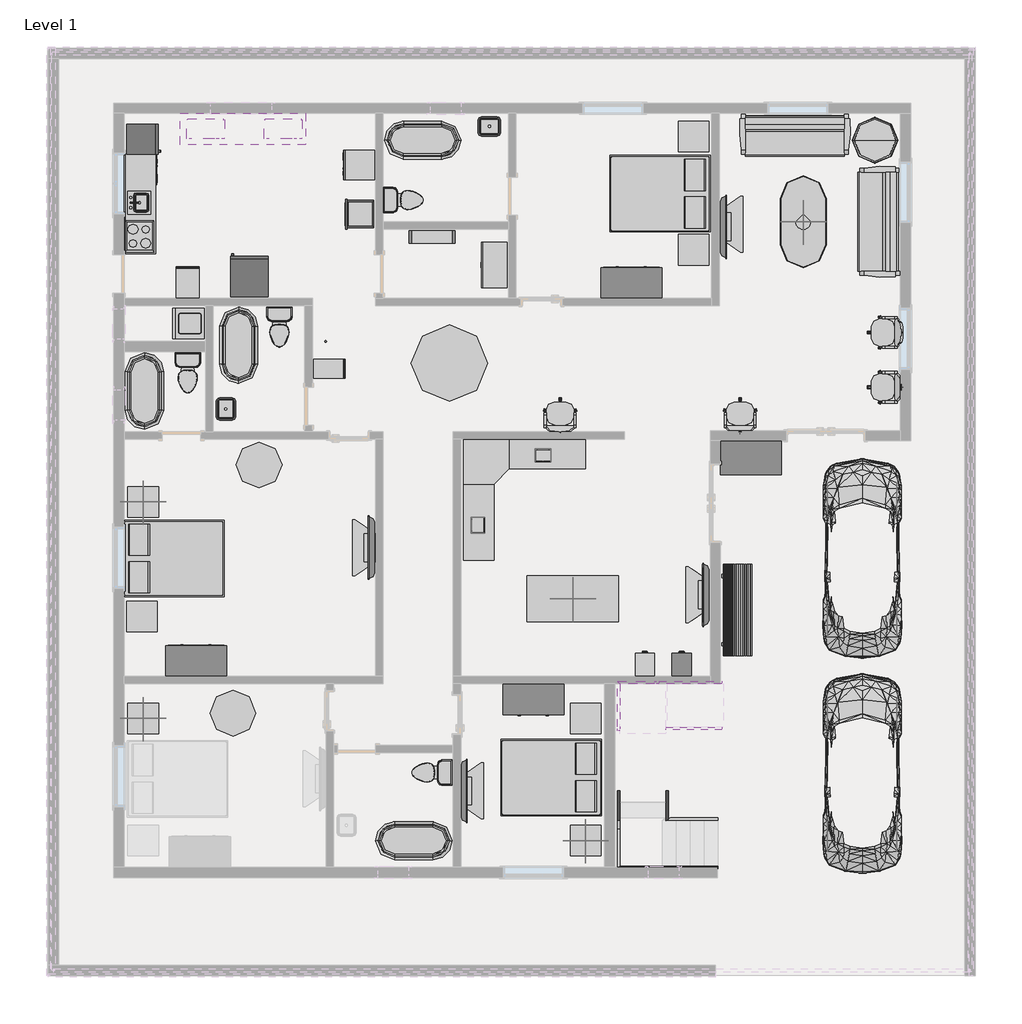
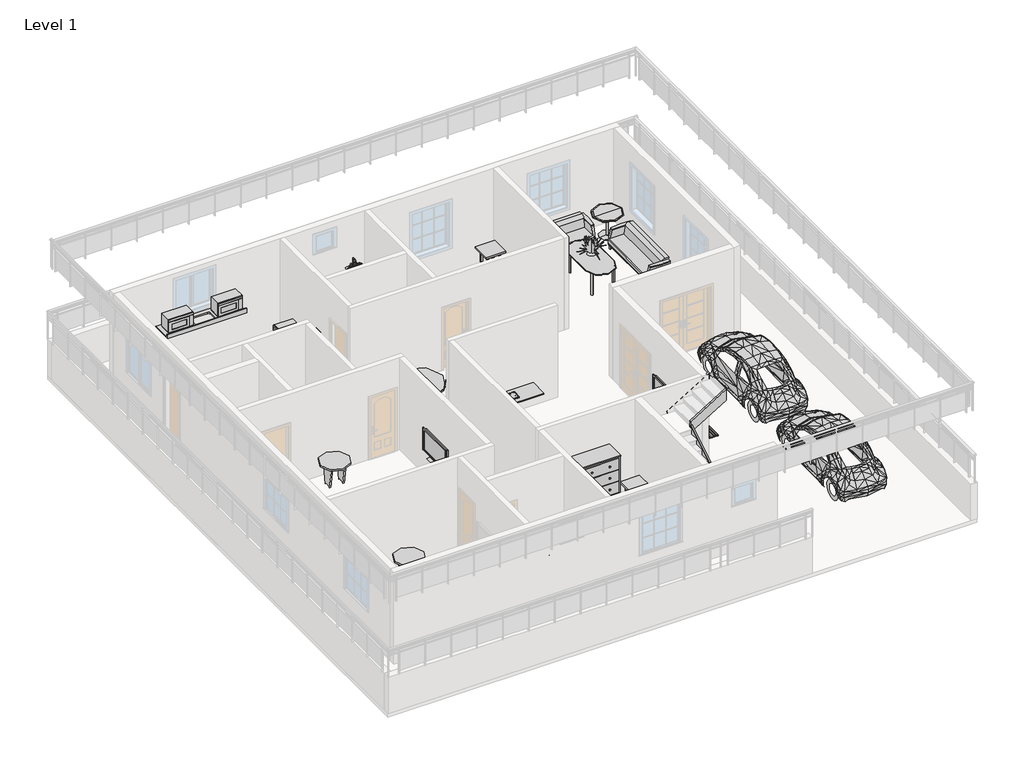
# One storey, part 6 of 6: 41 furniture elements, 16 proxies, 12 flow terminals, 10 members, 6 geographic elements.
"""IFC4 building model written with IfcOpenShell, lengths in millimetres."""

from ifc_helpers import new_model, si_unit, frame, origin, place, context, project, spatial, polyline, outline, extrude, faceted_brep, transform, mapped, element, save
from components import entourage_4c8cfd20, proxy_db4bb64d, proxy_7e1014cc, proxy_a6faaae8, proxy_53e5fb40, proxy_45b28599, kitchenette_medium_kitchenette_medium_844211aa, proxy_8a8d5ab2, proxy_8b8c2dc4, rpc_beetle_rpc_beetle_3ce7ba48, proxy_c523a7b7, proxy_a13a33b2, proxy_67057e99, flow_terminal_871c2e40, flow_terminal_d49f872f, flow_terminal_62a433f7, toilet_domestic_3d_toilet_domestic_3d_f7549cf7, toilet_domestic_3d_toilet_domestic_3d_183bbd19, flow_terminal_b374fae2, furniture_07436f11, furniture_1d2926bd, furniture_552c1472, furniture_b1353b55, chair_executive_chair_executive_8d69e98c, counter_top_w_sink_hole_0600mm_depth_f226a61d, furniture_c6510c7c, furniture_9fa109b2, furniture_80f2079a, furniture_417d203a, furniture_aff9b2fb, furniture_e1dba61b, furniture_fdf74506, tv_stand_tv_stand_6ce107e5, furniture_5644571f, furniture_2c34a4f9, furniture_bbcc68ce, furniture_4bee3317, furniture_5bc9ed15, furniture_c80d6d9c, geographic_element_235d1464, rpc_plant_tropical_agave_1_5_93a2a214

model = new_model("IFC4")

# Units and contexts
model_context = context("Model", 3, world=origin())
ifc_project = project(units=[si_unit("LENGTHUNIT", "METRE", prefix="MILLI")], contexts=[model_context])

# Site, building, storey
site = spatial("IfcSite", under=ifc_project)
building = spatial("IfcBuilding", under=site)
storey = spatial("IfcBuildingStorey", under=building, Name="Level 1", Elevation=0.0)

# Proxies
placement = place(None, origin())
entourage_shape = entourage_4c8cfd20(model_context)
element("IfcBuildingElementProxy", 1, Name="Entourage", at=placement, inside=storey, context=model_context, shape_type="MappedRepresentation", body=[
    mapped(entourage_shape, transform((1982.2015424, 5922.5758265, 762.0), x_axis=(1.0000000000000009, 0.0, 0.0), y_axis=(0.0, 1.0000000000000009, 0.0), z_axis=(0.0, 0.0, 1.0))),
])
element("IfcBuildingElementProxy", 2, Name="Entourage", at=placement, inside=storey, context=model_context, shape_type="MappedRepresentation", body=[
    mapped(entourage_shape, transform((644.6597674, 4493.3683542, 762.0), x_axis=(0.0, 1.0000000000000002, 0.0), y_axis=(-1.0000000000000002, 0.0, 0.0), z_axis=(0.0, 0.0, 1.0))),
])
proxy_shape = proxy_db4bb64d(model_context)
element("IfcBuildingElementProxy", 3, Name="15\" x 24\" x 34 1/2\"", ObjectType="15\" x 24\" x 34 1/2\"", at=placement, inside=storey, context=model_context, shape_type="MappedRepresentation", body=[
    mapped(proxy_shape, transform((-2024.5291533, 7343.658358, 0.0), x_axis=(0.0, 1.0000000000000002, 0.0), y_axis=(-1.0000000000000002, 0.0, 0.0), z_axis=(0.0, 0.0, 1.0))),
])
proxy_2_shape = proxy_7e1014cc(model_context)
element("IfcBuildingElementProxy", 4, Name="18\" x 24\" x 34 1/2\"", ObjectType="18\" x 24\" x 34 1/2\"", at=placement, inside=storey, context=model_context, shape_type="MappedRepresentation", body=[
    mapped(proxy_2_shape, transform((-4804.2612496, 9592.6253913, 0.0), x_axis=(-1.0000000000000004, 0.0, 0.0), y_axis=(0.0, -1.0000000000000004, 0.0), z_axis=(0.0, 0.0, 1.0))),
])
proxy_3_shape = proxy_a6faaae8(model_context)
element("IfcBuildingElementProxy", 5, Name="Cook Top-4 Unit2 : 22\" x 20\"", ObjectType="Cook Top-4 Unit2 : 22\" x 20\"", at=placement, inside=storey, context=model_context, shape_type="MappedRepresentation", body=[
    mapped(proxy_3_shape, transform((-6075.5787181, 10253.2758265, 0.0), x_axis=(0.0, 1.0000000000000002, 0.0), y_axis=(-1.0000000000000002, 0.0, 0.0), z_axis=(0.0, 0.0, 1.0))),
])
proxy_4_shape = proxy_53e5fb40(model_context)
element("IfcBuildingElementProxy", 6, Name="Dishwasher : 23\" x 23 11/16\" x 33 1/2\"", ObjectType="Dishwasher : 23\" x 23 11/16\" x 33 1/2\"", at=placement, inside=storey, context=model_context, shape_type="MappedRepresentation", body=[
    mapped(proxy_4_shape, transform((-1948.2710474, 12045.293295, 0.0), x_axis=(0.0, -1.0, 0.0), y_axis=(1.0, 0.0, 0.0), z_axis=(0.0, 0.0, 1.0))),
])
proxy_5_shape = proxy_45b28599(model_context)
element("IfcBuildingElementProxy", 7, Name="Dishwasher : 24\" x 24\" x 34\"", ObjectType="Dishwasher : 24\" x 24\" x 34\"", at=placement, inside=storey, context=model_context, shape_type="MappedRepresentation", body=[
    mapped(proxy_5_shape, transform((-5783.7291533, 11204.458358, 0.0), x_axis=(0.0, 1.0000000000000002, 0.0), y_axis=(-1.0000000000000002, 0.0, 0.0), z_axis=(0.0, 0.0, 1.0))),
])
kitchenette_medium_kitchenette_medium_shape = kitchenette_medium_kitchenette_medium_844211aa(model_context)
element("IfcBuildingElementProxy", 8, Name="Kitchenette - Medium : Kitchenette - Medium", ObjectType="Kitchenette - Medium : Kitchenette - Medium", at=placement, inside=storey, context=model_context, shape_type="MappedRepresentation", body=[
    mapped(kitchenette_medium_kitchenette_medium_shape, transform((-6380.3787181, 10577.4381216, 0.0), x_axis=(0.0, 1.0000000000000002, 0.0), y_axis=(-1.0000000000000002, 0.0, 0.0), z_axis=(0.0, 0.0, 1.0))),
])
proxy_6_shape = proxy_8a8d5ab2(model_context)
element("IfcBuildingElementProxy", 9, Name="Microwave : 30\" x 16\" x 18\"", ObjectType="Microwave : 30\" x 16\" x 18\"", at=placement, inside=storey, context=model_context, shape_type="MappedRepresentation", body=[
    mapped(proxy_6_shape, transform((-3705.6715955, 12754.2438323, 609.6), x_axis=(1.0000000000000007, 0.0, 0.0), y_axis=(0.0, 1.0000000000000007, 0.0), z_axis=(0.0, 0.0, 1.0))),
])
element("IfcBuildingElementProxy", 10, Name="Microwave : 30\" x 16\" x 18\"", ObjectType="Microwave : 30\" x 16\" x 18\"", at=placement, inside=storey, context=model_context, shape_type="MappedRepresentation", body=[
    mapped(proxy_6_shape, transform((-5255.0715955, 12754.2438323, 609.6), x_axis=(1.0000000000000004, 0.0, 0.0), y_axis=(0.0, 1.0000000000000004, 0.0), z_axis=(0.0, 0.0, 1.0))),
])
proxy_7_shape = proxy_8b8c2dc4(model_context)
element("IfcBuildingElementProxy", 11, Name="Oven Double-Built-in : 21 1/2\" x 39 1/4\" x 21\"", ObjectType="Oven Double-Built-in : 21 1/2\" x 39 1/4\" x 21\"", at=placement, inside=storey, context=model_context, shape_type="MappedRepresentation", body=[
    mapped(proxy_7_shape, transform((-1807.8060915, 10662.6008992, 0.0), x_axis=(0.0, -1.0, 0.0), y_axis=(1.0, 0.0, 0.0), z_axis=(0.0, 0.0, 1.0))),
])
rpc_beetle_rpc_beetle_shape = rpc_beetle_rpc_beetle_3ce7ba48(model_context)
element("IfcBuildingElementProxy", 12, Name="RPC Beetle : RPC Beetle", ObjectType="RPC Beetle : RPC Beetle", at=placement, inside=storey, context=model_context, shape_type="MappedRepresentation", body=[
    mapped(rpc_beetle_rpc_beetle_shape, transform((8351.6212819, 2595.1758265, 0.0), x_axis=(1.0, 0.0, 0.0), y_axis=(0.0, 1.0, 0.0), z_axis=(0.0, 0.0, 1.0))),
])
element("IfcBuildingElementProxy", 13, Name="RPC Beetle : RPC Beetle", ObjectType="RPC Beetle : RPC Beetle", at=placement, inside=storey, context=model_context, shape_type="MappedRepresentation", body=[
    mapped(rpc_beetle_rpc_beetle_shape, transform((8351.6212819, -1697.4241735, 0.0), x_axis=(1.0, 0.0, 0.0), y_axis=(0.0, 1.0, 0.0), z_axis=(0.0, 0.0, 1.0))),
])
proxy_8_shape = proxy_c523a7b7(model_context)
element("IfcBuildingElementProxy", 14, Name="Refrigerator : 24\" x 25\" LH", ObjectType="Refrigerator : 24\" x 25\" LH", at=placement, inside=storey, context=model_context, shape_type="MappedRepresentation", body=[
    mapped(proxy_8_shape, transform((-6029.9297466, 12190.0258265, 0.0), x_axis=(0.0, 1.0000000000000002, 0.0), y_axis=(-1.0000000000000002, 0.0, 0.0), z_axis=(0.0, 0.0, 1.0))),
])
proxy_9_shape = proxy_a13a33b2(model_context)
element("IfcBuildingElementProxy", 15, Name="Refrigerator : 30\" x 32\" RH", ObjectType="Refrigerator : 30\" x 32\" RH", at=placement, inside=storey, context=model_context, shape_type="MappedRepresentation", body=[
    mapped(proxy_9_shape, transform((-3883.2412181, 9439.276855, 0.0), x_axis=(-1.0000000000000004, 0.0, 0.0), y_axis=(0.0, -1.0000000000000004, 0.0), z_axis=(0.0, 0.0, 1.0))),
])
proxy_10_shape = proxy_67057e99(model_context)
element("IfcBuildingElementProxy", 16, Name="Washer : 27\" x 25\" x 35\"", ObjectType="Washer : 27\" x 25\" x 35\"", at=placement, inside=storey, context=model_context, shape_type="MappedRepresentation", body=[
    mapped(proxy_10_shape, transform((-4818.5291533, 8131.058358, 0.0), x_axis=(0.0, 1.0000000000000002, 0.0), y_axis=(-1.0000000000000002, 0.0, 0.0), z_axis=(0.0, 0.0, 1.0))),
])

# Flow terminals
flow_terminal_shape = flow_terminal_871c2e40(model_context)
element("IfcFlowTerminal", 17, ObjectType="Sink Kitchen-Island : 18\" x 18\"", at=placement, inside=storey, context=model_context, shape_type="MappedRepresentation", body=[
    mapped(flow_terminal_shape, transform((-6073.233317, 10910.6865859, -14.4), x_axis=(0.0, 1.0000000000000002, 0.0), y_axis=(-1.0000000000000002, 0.0, 0.0), z_axis=(0.0, 0.0, 1.0))),
])
flow_terminal_2_shape = flow_terminal_d49f872f(model_context)
element("IfcFlowTerminal", 18, ObjectType="Sink Vanity-Round : 19\" x 19\"", at=placement, inside=storey, context=model_context, shape_type="MappedRepresentation", body=[
    mapped(flow_terminal_2_shape, transform((-2272.1693735, 8061.1240859, 609.6), x_axis=(0.0, 1.0000000000000002, 0.0), y_axis=(-1.0000000000000002, 0.0, 0.0), z_axis=(0.0, 0.0, 1.0))),
])
flow_terminal_3_shape = flow_terminal_62a433f7(model_context)
element("IfcFlowTerminal", 19, ObjectType="Sink Vanity-Square : 20\" x 18\"", at=placement, inside=storey, context=model_context, shape_type="MappedRepresentation", body=[
    mapped(flow_terminal_3_shape, transform((-4403.183317, 6795.8865859, 609.6), x_axis=(0.0, 1.0, 0.0), y_axis=(-1.0, 0.0, 0.0), z_axis=(0.0, 0.0, 1.0))),
])
element("IfcFlowTerminal", 20, ObjectType="Sink Vanity-Square : 20\" x 18\"", at=placement, inside=storey, context=model_context, shape_type="MappedRepresentation", body=[
    mapped(flow_terminal_3_shape, transform((893.7320413, 12498.8304254, 609.6), x_axis=(1.0, 0.0, 0.0), y_axis=(0.0, 1.0, 0.0), z_axis=(0.0, 0.0, 1.0))),
])
toilet_domestic_3d_toilet_domestic_3d_shape = toilet_domestic_3d_toilet_domestic_3d_f7549cf7(model_context)
toilet_domestic_3d_toilet_domestic_3d_2_shape = toilet_domestic_3d_toilet_domestic_3d_183bbd19(model_context)
element("IfcFlowTerminal", 21, ObjectType="Toilet-Domestic-3D : Toilet-Domestic-3D", at=placement, inside=storey, context=model_context, shape_type="MappedRepresentation", body=[
    mapped(toilet_domestic_3d_toilet_domestic_3d_shape, transform((-714.8442052, 10977.1758265, 0.0), x_axis=(0.0, 1.0000000000000002, 0.0), y_axis=(-1.0000000000000002, 0.0, 0.0), z_axis=(0.0, 0.0, 1.0))),
    mapped(toilet_domestic_3d_toilet_domestic_3d_2_shape, transform((-714.8442052, 10977.1758265, 0.0), x_axis=(0.0, 1.0000000000000002, 0.0), y_axis=(-1.0000000000000002, 0.0, 0.0), z_axis=(0.0, 0.0, 1.0))),
])
element("IfcFlowTerminal", 22, ObjectType="Toilet-Domestic-3D : Toilet-Domestic-3D", at=placement, inside=storey, context=model_context, shape_type="MappedRepresentation", body=[
    mapped(toilet_domestic_3d_toilet_domestic_3d_shape, transform((-3281.5787181, 8348.8797992, 0.0), x_axis=(1.0, 0.0, 0.0), y_axis=(0.0, 1.0, 0.0), z_axis=(0.0, 0.0, 1.0))),
    mapped(toilet_domestic_3d_toilet_domestic_3d_2_shape, transform((-3281.5787181, 8348.8797992, 0.0), x_axis=(1.0, 0.0, 0.0), y_axis=(0.0, 1.0, 0.0), z_axis=(0.0, 0.0, 1.0))),
])
element("IfcFlowTerminal", 23, ObjectType="Toilet-Domestic-3D : Toilet-Domestic-3D", at=placement, inside=storey, context=model_context, shape_type="MappedRepresentation", body=[
    mapped(toilet_domestic_3d_toilet_domestic_3d_shape, transform((-5110.3787181, 7434.4797992, 0.0), x_axis=(1.0, 0.0, 0.0), y_axis=(0.0, 1.0, 0.0), z_axis=(0.0, 0.0, 1.0))),
    mapped(toilet_domestic_3d_toilet_domestic_3d_2_shape, transform((-5110.3787181, 7434.4797992, 0.0), x_axis=(1.0, 0.0, 0.0), y_axis=(0.0, 1.0, 0.0), z_axis=(0.0, 0.0, 1.0))),
])
element("IfcFlowTerminal", 24, ObjectType="Toilet-Domestic-3D : Toilet-Domestic-3D", at=placement, inside=storey, context=model_context, shape_type="MappedRepresentation", body=[
    mapped(toilet_domestic_3d_toilet_domestic_3d_shape, transform((-332.6362599, -441.2900026, 0.0), x_axis=(0.0, -1.0, 0.0), y_axis=(1.0, 0.0, 0.0), z_axis=(0.0, 0.0, 1.0))),
    mapped(toilet_domestic_3d_toilet_domestic_3d_2_shape, transform((-332.6362599, -441.2900026, 0.0), x_axis=(0.0, -1.0, 0.0), y_axis=(1.0, 0.0, 0.0), z_axis=(0.0, 0.0, 1.0))),
])
flow_terminal_4_shape = flow_terminal_b374fae2(model_context)
element("IfcFlowTerminal", 25, ObjectType="Tub-Free Standing-3D : 30\" x 60\"", at=placement, inside=storey, context=model_context, shape_type="MappedRepresentation", body=[
    mapped(flow_terminal_4_shape, transform((-5973.9787181, 7167.1758265, 0.0), x_axis=(1.0, 0.0, 0.0), y_axis=(0.0, 1.0, 0.0), z_axis=(0.0, 0.0, 1.0))),
])
element("IfcFlowTerminal", 26, ObjectType="Tub-Free Standing-3D : 30\" x 60\"", at=placement, inside=storey, context=model_context, shape_type="MappedRepresentation", body=[
    mapped(flow_terminal_4_shape, transform((-4094.3787181, 8081.5758265, 0.0), x_axis=(1.0, 0.0, 0.0), y_axis=(0.0, 1.0, 0.0), z_axis=(0.0, 0.0, 1.0))),
])
element("IfcFlowTerminal", 27, ObjectType="Tub-Free Standing-3D : 30\" x 60\"", at=placement, inside=storey, context=model_context, shape_type="MappedRepresentation", body=[
    mapped(flow_terminal_4_shape, transform((-422.1402326, 12170.9758265, 0.0), x_axis=(0.0, 1.0000000000000002, 0.0), y_axis=(-1.0000000000000002, 0.0, 0.0), z_axis=(0.0, 0.0, 1.0))),
])
element("IfcFlowTerminal", 28, ObjectType="Tub-Free Standing-3D : 30\" x 60\"", at=placement, inside=storey, context=model_context, shape_type="MappedRepresentation", body=[
    mapped(flow_terminal_4_shape, transform((-599.9402326, -1799.0241735, 0.0), x_axis=(0.0, -1.0, 0.0), y_axis=(1.0, 0.0, 0.0), z_axis=(0.0, 0.0, 1.0))),
])

# Furniture
furniture_shape = furniture_07436f11(model_context)
element("IfcFurniture", 29, ObjectType="96\" x 96\"", at=placement, inside=storey, context=model_context, shape_type="MappedRepresentation", body=[
    mapped(furniture_shape, transform((471.5915196, 6773.1988341, 0.0), x_axis=(1.0, 0.0, 0.0), y_axis=(0.0, 1.0, 0.0), z_axis=(0.0, 0.0, 1.0))),
])
furniture_2_shape = furniture_1d2926bd(model_context)
element("IfcFurniture", 30, ObjectType="Bed-Box : Queen 60\" x 79\"", at=placement, inside=storey, context=model_context, shape_type="MappedRepresentation", body=[
    mapped(furniture_2_shape, transform((-5624.2082263, 3487.9233675, 0.0), x_axis=(0.0, 1.0, 0.0), y_axis=(-1.0, 0.0, 0.0), z_axis=(0.0, 0.0, 1.0))),
])
element("IfcFurniture", 31, ObjectType="Bed-Box : Queen 60\" x 79\"", at=placement, inside=storey, context=model_context, shape_type="MappedRepresentation", body=[
    mapped(furniture_2_shape, transform((2377.6892756, -202.5717145, 0.0), x_axis=(0.0, -1.0, 0.0), y_axis=(1.0, 0.0, 0.0), z_axis=(0.0, 0.0, 1.0))),
])
element("IfcFurniture", 32, ObjectType="Bed-Box : Queen 60\" x 79\"", at=placement, inside=storey, context=model_context, shape_type="MappedRepresentation", body=[
    mapped(furniture_2_shape, transform((4549.3892756, 11443.3282855, 0.0), x_axis=(0.0, -1.0, 0.0), y_axis=(1.0, 0.0, 0.0), z_axis=(0.0, 0.0, 1.0))),
])
furniture_3_shape = furniture_552c1472(model_context)
element("IfcFurniture", 33, ObjectType="Cabinet-File 3 Drawer.0001 : 15\" x 18\"", at=placement, inside=storey, context=model_context, shape_type="MappedRepresentation", body=[
    mapped(furniture_3_shape, transform((3882.2633204, 1564.0415264, 0.0), x_axis=(-1.0, 0.0, 0.0), y_axis=(0.0, -1.0, 0.0), z_axis=(0.0, 0.0, 1.0))),
])
furniture_4_shape = furniture_b1353b55(model_context)
element("IfcFurniture", 34, ObjectType="Cabinet-File 4 Drawer : 15\" x 18\"", at=placement, inside=storey, context=model_context, shape_type="MappedRepresentation", body=[
    mapped(furniture_4_shape, transform((4618.8633204, 1564.0415264, 0.0), x_axis=(-1.0000000000000002, 0.0, 0.0), y_axis=(0.0, -1.0000000000000002, 0.0), z_axis=(0.0, 0.0, 1.0))),
])
chair_executive_chair_executive_shape = chair_executive_chair_executive_8d69e98c(model_context)
element("IfcFurniture", 35, ObjectType="Chair-Executive : Chair-Executive", at=placement, inside=storey, context=model_context, shape_type="MappedRepresentation", body=[
    mapped(chair_executive_chair_executive_shape, transform((8817.005669, 7102.3850068, 0.0), x_axis=(0.0, 1.0000000000000009, 0.0), y_axis=(-1.0000000000000009, 0.0, 0.0), z_axis=(0.0, 0.0, 1.0))),
])
element("IfcFurniture", 36, ObjectType="Chair-Executive : Chair-Executive", at=placement, inside=storey, context=model_context, shape_type="MappedRepresentation", body=[
    mapped(chair_executive_chair_executive_shape, transform((8817.005669, 8194.5850068, 0.0), x_axis=(0.0, 1.0000000000000002, 0.0), y_axis=(-1.0000000000000002, 0.0, 0.0), z_axis=(0.0, 0.0, 1.0))),
])
element("IfcFurniture", 37, ObjectType="Chair-Executive : Chair-Executive", at=placement, inside=storey, context=model_context, shape_type="MappedRepresentation", body=[
    mapped(chair_executive_chair_executive_shape, transform((5772.2304622, 6665.6299249, 0.0), x_axis=(1.0, 0.0, 0.0), y_axis=(0.0, 1.0, 0.0), z_axis=(0.0, 0.0, 1.0))),
])
element("IfcFurniture", 38, ObjectType="Chair-Executive : Chair-Executive", at=placement, inside=storey, context=model_context, shape_type="MappedRepresentation", body=[
    mapped(chair_executive_chair_executive_shape, transform((2180.0689477, 6665.6299249, 0.0), x_axis=(1.0, 0.0, 0.0), y_axis=(0.0, 1.0, 0.0), z_axis=(0.0, 0.0, 1.0))),
])
counter_top_w_sink_hole_0600mm_depth_shape = counter_top_w_sink_hole_0600mm_depth_f226a61d(model_context)
element("IfcFurniture", 39, ObjectType="Counter Top w Sink Hole : 0600mm Depth", at=placement, inside=storey, context=model_context, shape_type="MappedRepresentation", body=[
    mapped(counter_top_w_sink_hole_0600mm_depth_shape, transform((-3959.4025277, 12079.6945765, 609.6), x_axis=(-1.0, 0.0, 0.0), y_axis=(0.0, -1.0, 0.0), z_axis=(0.0, 0.0, 1.0))),
])
furniture_5_shape = furniture_c6510c7c(model_context)
element("IfcFurniture", 40, ObjectType="Counter Top w Sink Hole : 24\" Depth", at=placement, inside=storey, context=model_context, shape_type="MappedRepresentation", body=[
    mapped(furniture_5_shape, transform((-6380.3787181, 11110.8381216, -14.4), x_axis=(0.0, 1.0000000000000002, 0.0), y_axis=(-1.0000000000000002, 0.0, 0.0), z_axis=(0.0, 0.0, 1.0))),
])
furniture_6_shape = furniture_9fa109b2(model_context)
element("IfcFurniture", 41, ObjectType="Dresser : 48\" x 72\" x 24\"", at=placement, inside=storey, context=model_context, shape_type="MappedRepresentation", body=[
    mapped(furniture_6_shape, transform((-5212.5334924, 1419.2128724, 0.0), x_axis=(-1.0000000000000004, 0.0, 0.0), y_axis=(0.0, -1.0000000000000004, 0.0), z_axis=(0.0, 0.0, 1.0))),
])
element("IfcFurniture", 42, ObjectType="Dresser : 48\" x 72\" x 24\"", at=placement, inside=storey, context=model_context, shape_type="MappedRepresentation", body=[
    mapped(furniture_6_shape, transform((3474.2665076, 8963.0128724, 0.0), x_axis=(-1.0000000000000004, 0.0, 0.0), y_axis=(0.0, -1.0000000000000004, 0.0), z_axis=(0.0, 0.0, 1.0))),
])
element("IfcFurniture", 43, ObjectType="Dresser : 48\" x 72\" x 24\"", at=placement, inside=storey, context=model_context, shape_type="MappedRepresentation", body=[
    mapped(furniture_6_shape, transform((2056.8530272, 1383.5387806, 0.0), x_axis=(1.0, 0.0, 0.0), y_axis=(0.0, 1.0, 0.0), z_axis=(0.0, 0.0, 1.0))),
])
furniture_7_shape = furniture_80f2079a(model_context)
element("IfcFurniture", 44, ObjectType="Entertainment Center : 72\" x 72\" x 24\"", at=placement, inside=storey, context=model_context, shape_type="MappedRepresentation", body=[
    mapped(furniture_7_shape, transform((6131.0597674, 6278.1758265, 0.0), x_axis=(1.0, 0.0, 0.0), y_axis=(0.0, 1.0, 0.0), z_axis=(0.0, 0.0, 1.0))),
])
furniture_8_shape = furniture_417d203a(model_context)
element("IfcFurniture", 45, ObjectType="Shelving : 36\" x 10\" x 72\"", at=placement, inside=storey, context=model_context, shape_type="MappedRepresentation", body=[
    mapped(furniture_8_shape, transform((-233.5787181, 10545.3758265, 0.0), x_axis=(1.0, 0.0, 0.0), y_axis=(0.0, 1.0, 0.0), z_axis=(0.0, 0.0, 1.0))),
])
furniture_9_shape = furniture_aff9b2fb(model_context)
element("IfcFurniture", 46, ObjectType="Sofa-Pensi : 84\"", at=placement, inside=storey, context=model_context, shape_type="MappedRepresentation", body=[
    mapped(furniture_9_shape, transform((6726.8150319, 11989.1159904, 0.0), x_axis=(1.0, 0.0, 0.0), y_axis=(0.0, 1.0, 0.0), z_axis=(0.0, 0.0, 1.0))),
])
element("IfcFurniture", 47, ObjectType="Sofa-Pensi : 84\"", at=placement, inside=storey, context=model_context, shape_type="MappedRepresentation", body=[
    mapped(furniture_9_shape, transform((8404.7114458, 10823.9820765, 0.0), x_axis=(0.0, -1.0000000000000004, 0.0), y_axis=(1.0000000000000004, 0.0, 0.0), z_axis=(0.0, 0.0, 1.0))),
])
furniture_10_shape = furniture_e1dba61b(model_context)
element("IfcFurniture", 48, ObjectType="Storage Pedestal : 20\" x 36\" x 36\"", at=placement, inside=storey, context=model_context, shape_type="MappedRepresentation", body=[
    mapped(furniture_10_shape, transform((1945.3396579, 9501.7533126, 0.0), x_axis=(0.0, -1.0000000000000004, 0.0), y_axis=(1.0000000000000004, 0.0, 0.0), z_axis=(0.0, 0.0, 1.0))),
])
furniture_11_shape = furniture_fdf74506(model_context)
element("IfcFurniture", 49, ObjectType="TV - Flat Screen : 50\"", at=placement, inside=storey, context=model_context, shape_type="MappedRepresentation", body=[
    mapped(furniture_11_shape, transform((-1440.4689881, 4039.0313124, 914.4), x_axis=(0.0, -1.0, 0.0), y_axis=(1.0, 0.0, 0.0), z_axis=(0.0, 0.0, 1.0))),
])
element("IfcFurniture", 50, ObjectType="TV - Flat Screen : 50\"", at=placement, inside=storey, context=model_context, shape_type="MappedRepresentation", body=[
    mapped(furniture_11_shape, transform((398.3983911, -804.4796594, 914.4), x_axis=(0.0, 1.0000000000000002, 0.0), y_axis=(-1.0000000000000002, 0.0, 0.0), z_axis=(0.0, 0.0, 1.0))),
])
element("IfcFurniture", 51, ObjectType="TV - Flat Screen : 50\"", at=placement, inside=storey, context=model_context, shape_type="MappedRepresentation", body=[
    mapped(furniture_11_shape, transform((5234.3211438, 3099.2313124, 914.4), x_axis=(0.0, -1.0000000000000004, 0.0), y_axis=(1.0000000000000004, 0.0, 0.0), z_axis=(0.0, 0.0, 1.0))),
])
element("IfcFurniture", 52, ObjectType="TV - Flat Screen : 50\"", at=placement, inside=storey, context=model_context, shape_type="MappedRepresentation", body=[
    mapped(furniture_11_shape, transform((5573.6483911, 10447.7203406, 914.4), x_axis=(0.0, 1.0000000000000002, 0.0), y_axis=(-1.0000000000000002, 0.0, 0.0), z_axis=(0.0, 0.0, 1.0))),
])
tv_stand_tv_stand_shape = tv_stand_tv_stand_6ce107e5(model_context)
element("IfcFurniture", 53, ObjectType="TV Stand : TV Stand", at=placement, inside=storey, context=model_context, shape_type="MappedRepresentation", body=[
    mapped(tv_stand_tv_stand_shape, transform((-1361.9402326, 4168.1638286, 0.0), x_axis=(0.0, -1.0000000000000004, 0.0), y_axis=(1.0000000000000004, 0.0, 0.0), z_axis=(0.0, 0.0, 1.0))),
])
element("IfcFurniture", 54, ObjectType="TV Stand : TV Stand", at=placement, inside=storey, context=model_context, shape_type="MappedRepresentation", body=[
    mapped(tv_stand_tv_stand_shape, transform((339.8597674, -933.6121756, 0.0), x_axis=(0.0, 1.0000000000000002, 0.0), y_axis=(-1.0000000000000002, 0.0, 0.0), z_axis=(0.0, 0.0, 1.0))),
])
element("IfcFurniture", 55, ObjectType="TV Stand : TV Stand", at=placement, inside=storey, context=model_context, shape_type="MappedRepresentation", body=[
    mapped(tv_stand_tv_stand_shape, transform((5292.8597674, 3228.3638286, 0.0), x_axis=(0.0, -1.0000000000000004, 0.0), y_axis=(1.0000000000000004, 0.0, 0.0), z_axis=(0.0, 0.0, 1.0))),
])
element("IfcFurniture", 56, ObjectType="TV Stand : TV Stand", at=placement, inside=storey, context=model_context, shape_type="MappedRepresentation", body=[
    mapped(tv_stand_tv_stand_shape, transform((5515.1097674, 10369.3878244, 0.0), x_axis=(0.0, 1.0000000000000002, 0.0), y_axis=(-1.0000000000000002, 0.0, 0.0), z_axis=(0.0, 0.0, 1.0))),
])
furniture_12_shape = furniture_5644571f(model_context)
element("IfcFurniture", 57, ObjectType="Table-Dining : 24\" x 36\" x 24\"", at=placement, inside=storey, context=model_context, shape_type="MappedRepresentation", body=[
    mapped(furniture_12_shape, transform((2556.7940007, 2931.7647487, 0.0), x_axis=(1.0, 0.0, 0.0), y_axis=(0.0, 1.0, 0.0), z_axis=(0.0, 0.0, 1.0))),
])
furniture_13_shape = furniture_2c34a4f9(model_context)
element("IfcFurniture", 58, ObjectType="Table-Dining Oval : 36\" x 72\"", at=placement, inside=storey, context=model_context, shape_type="MappedRepresentation", body=[
    mapped(furniture_13_shape, transform((6814.3614068, 10947.1954986, 0.0), x_axis=(0.0, 1.0, 0.0), y_axis=(-1.0, 0.0, 0.0), z_axis=(0.0, 0.0, 1.0))),
])
furniture_14_shape = furniture_bbcc68ce(model_context)
element("IfcFurniture", 59, ObjectType="Table-Dining Round w Chairs : 60\" Diameter", at=placement, inside=storey, context=model_context, shape_type="MappedRepresentation", body=[
    mapped(furniture_14_shape, transform((7.5778002, 7910.854515, 0.0), x_axis=(1.0, 0.0, 0.0), y_axis=(0.0, 1.0, 0.0), z_axis=(0.0, 0.0, 1.0))),
])
furniture_15_shape = furniture_4bee3317(model_context)
element("IfcFurniture", 60, ObjectType="Table-Ellipse : 72\" x 36\"", at=placement, inside=storey, context=model_context, shape_type="MappedRepresentation", body=[
    mapped(furniture_15_shape, transform((-3687.9787181, 5693.9758265, 0.0), x_axis=(1.0, 0.0, 0.0), y_axis=(0.0, 1.0, 0.0), z_axis=(0.0, 0.0, 1.0))),
])
element("IfcFurniture", 61, ObjectType="Table-Ellipse : 72\" x 36\"", at=placement, inside=storey, context=model_context, shape_type="MappedRepresentation", body=[
    mapped(furniture_15_shape, transform((-4208.3632197, 742.8480226, 0.0), x_axis=(1.0, 0.0, 0.0), y_axis=(0.0, 1.0, 0.0), z_axis=(0.0, 0.0, 1.0))),
])
furniture_16_shape = furniture_5bc9ed15(model_context)
element("IfcFurniture", 62, ObjectType="Table-Night Stand : 24\" x 24\" x 30\"", at=placement, inside=storey, context=model_context, shape_type="MappedRepresentation", body=[
    mapped(furniture_16_shape, transform((-6307.9123484, 334.5758265, 0.0), x_axis=(1.0, 0.0, 0.0), y_axis=(0.0, 1.0, 0.0), z_axis=(0.0, 0.0, 1.0))),
])
element("IfcFurniture", 63, ObjectType="Table-Night Stand : 24\" x 24\" x 30\"", at=placement, inside=storey, context=model_context, shape_type="MappedRepresentation", body=[
    mapped(furniture_16_shape, transform((2520.5261371, -2103.8241735, 0.0), x_axis=(1.0, 0.0, 0.0), y_axis=(0.0, 1.0, 0.0), z_axis=(0.0, 0.0, 1.0))),
])
element("IfcFurniture", 64, ObjectType="Table-Night Stand : 24\" x 24\" x 30\"", at=placement, inside=storey, context=model_context, shape_type="MappedRepresentation", body=[
    mapped(furniture_16_shape, transform((2520.5261371, 334.5758265, 0.0), x_axis=(1.0, 0.0, 0.0), y_axis=(0.0, 1.0, 0.0), z_axis=(0.0, 0.0, 1.0))),
])
element("IfcFurniture", 65, ObjectType="Table-Night Stand : 24\" x 24\" x 30\"", at=placement, inside=storey, context=model_context, shape_type="MappedRepresentation", body=[
    mapped(furniture_16_shape, transform((-6333.3123484, 2366.5758265, 0.0), x_axis=(1.0, 0.0, 0.0), y_axis=(0.0, 1.0, 0.0), z_axis=(0.0, 0.0, 1.0))),
])
element("IfcFurniture", 66, ObjectType="Table-Night Stand : 24\" x 24\" x 30\"", at=placement, inside=storey, context=model_context, shape_type="MappedRepresentation", body=[
    mapped(furniture_16_shape, transform((-6307.9123484, 4652.5758265, 0.0), x_axis=(1.0, 0.0, 0.0), y_axis=(0.0, 1.0, 0.0), z_axis=(0.0, 0.0, 1.0))),
])
element("IfcFurniture", 67, ObjectType="Table-Night Stand : 24\" x 24\" x 30\"", at=placement, inside=storey, context=model_context, shape_type="MappedRepresentation", body=[
    mapped(furniture_16_shape, transform((4679.5261371, 11942.3758265, 0.0), x_axis=(1.0, 0.0, 0.0), y_axis=(0.0, 1.0, 0.0), z_axis=(0.0, 0.0, 1.0))),
])
element("IfcFurniture", 68, ObjectType="Table-Night Stand : 24\" x 24\" x 30\"", at=placement, inside=storey, context=model_context, shape_type="MappedRepresentation", body=[
    mapped(furniture_16_shape, transform((4679.5261371, 9681.7758265, 0.0), x_axis=(1.0, 0.0, 0.0), y_axis=(0.0, 1.0, 0.0), z_axis=(0.0, 0.0, 1.0))),
])
furniture_17_shape = furniture_c80d6d9c(model_context)
element("IfcFurniture", 69, ObjectType="Table-Round : 36\" Diameter", at=placement, inside=storey, context=model_context, shape_type="MappedRepresentation", body=[
    mapped(furniture_17_shape, transform((8605.6212819, 12170.9758265, 0.0), x_axis=(1.0, 0.0, 0.0), y_axis=(0.0, 1.0, 0.0), z_axis=(0.0, 0.0, 1.0))),
])

# Geographic elements
geographic_element_shape = geographic_element_235d1464(model_context)
element("IfcGeographicElement", 70, ObjectType="Park Bench : 72\"", at=placement, inside=storey, context=model_context, shape_type="MappedRepresentation", body=[
    mapped(geographic_element_shape, transform((5826.2597674, 2798.3758265, 0.0), x_axis=(0.0, 1.0000000000000002, 0.0), y_axis=(-1.0000000000000002, 0.0, 0.0), z_axis=(0.0, 0.0, 1.0))),
])
rpc_plant_tropical_agave_1_5_shape = rpc_plant_tropical_agave_1_5_93a2a214(model_context)
element("IfcGeographicElement", 71, ObjectType="RPC Plant - Tropical : Agave - 1.5'", at=placement, inside=storey, context=model_context, shape_type="MappedRepresentation", body=[
    mapped(rpc_plant_tropical_agave_1_5_shape, transform((2575.0597674, 3026.9758265, 609.6), x_axis=(1.0, 0.0, 0.0), y_axis=(0.0, 1.0, 0.0), z_axis=(0.0, 0.0, 1.0))),
])
element("IfcGeographicElement", 72, ObjectType="RPC Plant - Tropical : Agave - 1.5'", at=placement, inside=storey, context=model_context, shape_type="MappedRepresentation", body=[
    mapped(rpc_plant_tropical_agave_1_5_shape, transform((7172.4597674, 10545.3758265, 914.4), x_axis=(1.0, 0.0, 0.0), y_axis=(0.0, 1.0, 0.0), z_axis=(0.0, 0.0, 1.0))),
])
element("IfcGeographicElement", 73, ObjectType="RPC Plant - Tropical : Agave - 1.5'", at=placement, inside=storey, context=model_context, shape_type="MappedRepresentation", body=[
    mapped(rpc_plant_tropical_agave_1_5_shape, transform((-5999.3787181, 4957.3758265, 762.0), x_axis=(1.0, 0.0, 0.0), y_axis=(0.0, 1.0, 0.0), z_axis=(0.0, 0.0, 1.0))),
])
element("IfcGeographicElement", 74, ObjectType="RPC Plant - Tropical : Agave - 1.5'", at=placement, inside=storey, context=model_context, shape_type="MappedRepresentation", body=[
    mapped(rpc_plant_tropical_agave_1_5_shape, transform((-5999.3787181, 639.3758265, 762.0), x_axis=(1.0, 0.0, 0.0), y_axis=(0.0, 1.0, 0.0), z_axis=(0.0, 0.0, 1.0))),
])
element("IfcGeographicElement", 75, ObjectType="RPC Plant - Tropical : Agave - 1.5'", at=placement, inside=storey, context=model_context, shape_type="MappedRepresentation", body=[
    mapped(rpc_plant_tropical_agave_1_5_shape, transform((2829.0597674, -1799.0241735, 762.0), x_axis=(1.0, 0.0, 0.0), y_axis=(0.0, 1.0, 0.0), z_axis=(0.0, 0.0, 1.0))),
])

# Members
element("IfcMember", 76, ObjectType="Stringer - 2\" Width", at=placement, inside=storey, context=model_context, shape_type="SweptSolid", body=[
    extrude(outline(polyline([(25.0390838, 5470.6597674), (381.4478453, 5470.6597674), (1092.2, 4297.9187121), (787.4, 4212.7642556), (25.0390838, 5470.6597674)])), frame((0.0, -2357.8241735, 0.0), z_axis=(0.0, 1.0, 0.0), x_axis=(0.0, 0.0, 1.0)), (0.0, 0.0, 1.0), 50.8),
])
element("IfcMember", 77, ObjectType="Stringer - 2\" Width", at=placement, inside=storey, context=model_context, shape_type="Brep", body=[
    faceted_brep([(5470.6597674, -1341.8241735, 381.4478453), (5470.6597674, -1392.6241735, 381.4478453), (5470.6597674, -1392.6241735, 25.0390838), (5470.6597674, -1341.8241735, 25.0390838), (4520.8407698, -1341.8241735, 957.0957226), (4444.6407698, -1392.6241735, 1003.2775408), (4444.6407698, -1392.6241735, 646.8687793), (4520.8407698, -1341.8241735, 600.6869611)], [[[0, 1, 2, 3]], [[1, 0, 4, 5]], [[2, 1, 5, 6]], [[3, 2, 6, 7]], [[0, 3, 7, 4]], [[4, 7, 6, 5]]]),
])
element("IfcMember", 78, ObjectType="Stringer - 2\" Width", at=placement, inside=storey, context=model_context, shape_type="SweptSolid", body=[
    extrude(outline(polyline([(-1480.9286617, 787.4), (-1566.0831182, 1092.2), (389.7168818, 2277.5333333), (474.8713383, 1972.7333333), (-1480.9286617, 787.4)])), frame((3464.0597674, 0.0, 0.0), z_axis=(1.0, 0.0, 0.0), x_axis=(0.0, 1.0, 0.0)), (0.0, 0.0, 1.0), 50.8),
])
element("IfcMember", 79, ObjectType="Stringer - 2\" Width", at=placement, inside=storey, context=model_context, shape_type="Brep", body=[
    faceted_brep([(4429.2597674, -1402.8781751, 1191.1120868), (4480.0597674, -1369.0115084, 1211.6373393), (4480.0597674, 410.7758265, 2290.2963301), (4429.2597674, 410.7758265, 2290.2963301), (4429.2597674, -1402.8781751, 834.7033252), (4429.2597674, 410.7758265, 1933.8875686), (4480.0597674, -1369.0115084, 855.2285778), (4480.0597674, 410.7758265, 1933.8875686)], [[[0, 1, 2, 3]], [[4, 0, 3, 5]], [[6, 4, 5, 7]], [[1, 6, 7, 2]], [[1, 0, 4, 6]], [[2, 7, 5, 3]]]),
])
element("IfcMember", 80, ObjectType="Stringer - 2\" Width", at=placement, inside=storey, context=model_context, shape_type="Brep", body=[
    faceted_brep([(3514.8597674, -1566.0831182, 1092.2), (3464.0597674, -1566.0831182, 1092.2), (3464.0597674, -2357.8241735, 1092.2), (3514.8597674, -2307.0241735, 1092.2), (3514.8597674, -1480.9286617, 787.4), (3514.8597674, -2307.0241735, 787.4), (3464.0597674, -1480.9286617, 787.4), (3464.0597674, -2357.8241735, 787.4)], [[[0, 1, 2, 3]], [[4, 0, 3, 5]], [[6, 4, 5, 7]], [[1, 6, 7, 2]], [[1, 0, 4, 6]], [[2, 7, 5, 3]]]),
])
element("IfcMember", 81, ObjectType="Stringer - 2\" Width", at=placement, inside=storey, context=model_context, shape_type="Brep", body=[
    faceted_brep([(3514.8597674, -2307.0241735, 1092.2), (3464.0597674, -2357.8241735, 1092.2), (4297.9187121, -2357.8241735, 1092.2), (4297.9187121, -2307.0241735, 1092.2), (3514.8597674, -2307.0241735, 787.4), (4212.7642556, -2307.0241735, 787.4), (3464.0597674, -2357.8241735, 787.4), (4212.7642556, -2357.8241735, 787.4)], [[[0, 1, 2, 3]], [[4, 0, 3, 5]], [[6, 4, 5, 7]], [[1, 6, 7, 2]], [[1, 0, 4, 6]], [[2, 7, 5, 3]]]),
])
element("IfcMember", 82, ObjectType="Stringer - 2\" Width", at=placement, inside=storey, context=model_context, shape_type="SweptSolid", body=[
    extrude(outline(polyline([(2277.5333333, 4205.0008227), (1972.7333333, 4290.1552792), (2734.3724171, 5546.8597674), (3090.7811786, 5546.8597674), (2277.5333333, 4205.0008227)])), frame((0.0, 1325.1758265, 0.0), z_axis=(0.0, 1.0, 0.0), x_axis=(0.0, 0.0, 1.0)), (0.0, 0.0, 1.0), 50.8),
])
element("IfcMember", 83, ObjectType="Stringer - 2\" Width", at=placement, inside=storey, context=model_context, shape_type="SweptSolid", body=[
    extrude(outline(polyline([(2413.4478453, 4429.2597674), (2057.0390838, 4429.2597674), (2734.3724171, 5546.8597674), (3090.7811786, 5546.8597674), (2413.4478453, 4429.2597674)])), frame((0.0, 410.7758265, 0.0), z_axis=(0.0, 1.0, 0.0), x_axis=(0.0, 0.0, 1.0)), (0.0, 0.0, 1.0), 50.8),
])
element("IfcMember", 84, ObjectType="Stringer - 2\" Width", at=placement, inside=storey, context=model_context, shape_type="Brep", body=[
    faceted_brep([(4205.0008227, 1325.1758265, 2277.5333333), (4205.0008227, 1375.9758265, 2277.5333333), (3464.0597674, 1375.9758265, 2277.5333333), (3514.8597674, 1325.1758265, 2277.5333333), (4290.1552792, 1325.1758265, 1972.7333333), (3514.8597674, 1325.1758265, 1972.7333333), (4290.1552792, 1375.9758265, 1972.7333333), (3464.0597674, 1375.9758265, 1972.7333333)], [[[0, 1, 2, 3]], [[4, 0, 3, 5]], [[6, 4, 5, 7]], [[1, 6, 7, 2]], [[2, 7, 5, 3]], [[1, 0, 4, 6]]]),
])
element("IfcMember", 85, ObjectType="Stringer - 2\" Width", at=placement, inside=storey, context=model_context, shape_type="Brep", body=[
    faceted_brep([(3514.8597674, 1325.1758265, 2277.5333333), (3464.0597674, 1375.9758265, 2277.5333333), (3464.0597674, 389.7168818, 2277.5333333), (3514.8597674, 389.7168818, 2277.5333333), (3514.8597674, 1325.1758265, 1972.7333333), (3514.8597674, 474.8713383, 1972.7333333), (3464.0597674, 1375.9758265, 1972.7333333), (3464.0597674, 474.8713383, 1972.7333333)], [[[0, 1, 2, 3]], [[4, 0, 3, 5]], [[6, 4, 5, 7]], [[1, 6, 7, 2]], [[1, 0, 4, 6]], [[2, 7, 5, 3]]]),
])

save(model, "model.ifc")

# Revit data of these elements
# Type
#   built-in parameter 1005195 = "RPC-16-N04H-AQSP-D1N4-43SU-6GKQ-C3KU-1C"
#   Height = 0
# Type "15\" x 24\" x 34 1/2\""
#   Label = "T"
#   Assembly Code = "E1090400"
#   Depth = 2' - 0"
#   Height = 2' - 10 1/2"
#   Width = 1' - 3"
#   Panel Face Material = Plastic, Opaque Black
#   Trach Compact. Material = Steel, Paint Finish, Ivory, Matte
#   Default Elevation = 0
# Type "18\" x 24\" x 34 1/2\""
#   Label = "T"
#   Assembly Code = "E1090400"
#   Depth = 2' - 0"
#   Height = 2' - 10 1/2"
#   Width = 1' - 6"
#   Panel Face Material = Plastic, Opaque Black
#   Trach Compact. Material = Steel, Paint Finish, Ivory, Matte
#   Default Elevation = 0
# Type "Cook Top-4 Unit2 : 22\" x 20\""
#   Depth = 1' - 8"
#   Width = 1' - 10"
#   Burner Material = Steel, Chrome Plated
#   Cooktop Material = Steel, Polished
#   Default Elevation = 0
#   Assembly Code = ""
# Type "Dishwasher : 23\" x 23 11/16\" x 33 1/2\""
#   Label = "DW"
#   Assembly Code = "E1090400"
#   Depth = 1' - 11 11/16"
#   Height = 2' - 9 1/2"
#   Width = 1' - 11"
#   Dishwasher Material = Steel, Paint Finish, Ivory, Glossy
#   Panel Face Material = Plastic, Opaque Black
#   Default Elevation = 0
# Type "Dishwasher : 24\" x 24\" x 34\""
#   Label = "DW"
#   Assembly Code = "E1090400"
#   Depth = 2' - 0"
#   Height = 2' - 10"
#   Width = 2' - 0"
#   Dishwasher Material = Steel, Paint Finish, Ivory, Glossy
#   Panel Face Material = Plastic, Opaque Black
#   Default Elevation = 0
# Type "Kitchenette - Medium : Kitchenette - Medium"
#   Assembly Code = "E1090400"
#   Counter Length = 6' - 6"
#   Cabinet Width = 4' - 6"
#   Cabinet Height = 2' - 10 1/2"
#   Cabinet Depth = 2' - 0"
#   Toe Depth = 0' - 3"
#   Toe Height = 0' - 3 1/2"
#   Cabinet Material = Cabinets
#   Door/Drawer Material = Cabinets
#   Handle Material = Cabinets - Handles
#   Default Elevation = 0
# Type "Microwave : 30\" x 16\" x 18\""
#   Assembly Code = "E1090400"
#   Depth = 1' - 4"
#   Height = 1' - 6"
#   Width = 2' - 6"
#   Microwave Material = Laminate, Ivory, Matte
#   Default Elevation = 0
# Type "Oven Double-Built-in : 21 1/2\" x 39 1/4\" x 21\""
#   Label = "OVEN"
#   Assembly Code = "E1090400"
#   Depth = 1' - 9"
#   Height = 3' - 3 1/4"
#   Width = 1' - 9 1/2"
#   Oven Material = Metal - Stainless Steel, Polished
#   Default Elevation = 0
# Type "RPC Beetle : RPC Beetle"
#   built-in parameter 1005195 = "RPC-16-0U6E-L4EG-ENH1-J3KF-SVEL-0TX4-C0"
#   Height = 0
# Type "Refrigerator : 24\" x 25\" LH"
#   Label = "REF."
#   Assembly Code = "E1090400"
#   Depth = 2' - 0 3/4"
#   Handle = 0' - 1 1/2"
#   Height = 5' - 3 1/2"
#   Rear Clearance = 0' - 2"
#   Top Door Height = 1' - 8"
#   Width = 1' - 11 1/2"
#   Material = Steel, Paint Finish, Ivory, Glossy
#   Default Elevation = 0
# Type "Refrigerator : 30\" x 32\" RH"
#   Label = "REF."
#   Assembly Code = "E1090400"
#   Depth = 2' - 7 3/4"
#   Handle = 2' - 3"
#   Height = 5' - 10"
#   Rear Clearance = 0' - 2"
#   Top Door Height = 1' - 8"
#   Width = 2' - 5 3/8"
#   Material = Steel, Paint Finish, Ivory, Glossy
#   Default Elevation = 0
# Type "Washer : 27\" x 25\" x 35\""
#   Label = "W"
#   Assembly Code = "E1090400"
#   Depth = 2' - 1"
#   Height = 2' - 11"
#   Width = 2' - 0"
#   Washer Material = Steel, Paint Finish, Ivory, Matte
#   Default Elevation = 0
# Type "Sink Kitchen-Island : 18\" x 18\""
#   Assembly Code = "D2010410"
#   Counter Height = 3' - 0"
#   Depth = 1' - 6"
#   Width = 1' - 6"
#   Faucet Material = Steel, Polished
#   Sink Material = Steel, Polished
#   Default Elevation = 0
# Type "Sink Vanity-Round : 19\" x 19\""
#   Assembly Code = "D2010400"
#   Top Of Counter = 2' - 7"
#   Basin Material = Porcelain, Linen
#   Faucet Material = Steel, Polished
#   Default Elevation = 0
# Type "Sink Vanity-Square : 20\" x 18\""
#   Assembly Code = "D2010400"
#   Counter Height = 2' - 7"
#   Depth = 1' - 6"
#   Width = 1' - 8"
#   Basin Material = Porcelain, Linen
#   Faucet Material = Steel, Polished
#   Default Elevation = 0
# Type "Toilet-Domestic-3D : Toilet-Domestic-3D"
#   Assembly Code = "D2010110"
#   Toilet - Bowl/Basin Material = Porcelain, Linen
#   Toilet - Seat Material = Laminate, Linen, Matte
#   Default Elevation = 0
# Type "Tub-Free Standing-3D : 30\" x 60\""
#   Assembly Code = "D2010110"
#   Height = 1' - 6"
#   Length = 5' - 0"
#   Width = 2' - 6"
#   Tub Material = Porcelain, Ivory
#   Default Elevation = 0
# Type "96\" x 96\""
#   Assembly Code = "E2020"
#   Desktop Height = 2' - 6"
#   Desktop1 Width = 2' - 0"
#   Desktop2 Width = 2' - 0"
#   Panel1 Length = 5' - 0"
#   Panel2 Length = 5' - 0"
#   Work Top Material = Laminate, Ivory, Matte
#   Default Elevation = 0
# Type "Bed-Box : Queen 60\" x 79\""
#   Assembly Code = "E2020200"
#   Length = 6' - 7"
#   Width = 5' - 0"
#   Frame Material = Birch
#   Mattress Material = Linen, White
#   Default Elevation = 0
# Type "Cabinet-File 3 Drawer.0001 : 15\" x 18\""
#   Assembly Code = "E2020200"
#   Depth = 1' - 6"
#   Height = 3' - 5"
#   Width = 1' - 3"
#   Cabinet Material = Steel, Paint Finish, Ivory, Glossy
#   Handle Material = Steel, Chrome Plated
#   Default Elevation = 0
# Type "Cabinet-File 4 Drawer : 15\" x 18\""
#   Assembly Code = "E2020200"
#   Depth = 1' - 6"
#   Height = 4' - 4"
#   Width = 1' - 3"
#   Cabinet Material = Steel, Paint Finish, Ivory, Glossy
#   Handle Material = Steel, Chrome Plated
#   Default Elevation = 0
# Type "Chair-Executive : Chair-Executive"
#   Assembly Code = "E2020200"
#   Base/Arms Material = Plastic, Opaque Black
#   Casters Material = Plastic, Opaque Black
#   Seat/Back Material = Textile - Slate Blue
#   Default Elevation = 0
# Type "Counter Top w Sink Hole : 0600mm Depth"
#   Assembly Code = "C1030400"
#   Counter Thickness = 0' - 1 9/16"
#   Depth = 2' - 0 19/32"
#   Height = 2' - 11 7/16"
#   Length [instance default] = 8' - 2 7/16"
#   Sink Location [instance default] = 3' - 11 1/4"
#   Sink Location To Wall [instance default] = 0' - 3 15/16"
#   Sink Opening Depth [instance default] = 1' - 2 7/8"
#   Sink Opening Width [instance default] = 1' - 11 1/8"
#   Counter Top Material = none
#   Default Elevation = 0
# Type "Counter Top w Sink Hole : 24\" Depth"
#   Assembly Code = "C1030400"
#   Counter Thickness = 0' - 1 1/2"
#   Depth = 2' - 1"
#   Height = 3' - 0"
#   Length [instance default] = 8' - 0"
#   Sink Location [instance default] = 2' - 0"
#   Sink Location To Wall [instance default] = 0' - 6"
#   Sink Opening Depth [instance default] = 1' - 3"
#   Sink Opening Width [instance default] = 2' - 3"
#   Counter Top Material = none
#   Default Elevation = 0
# Type "Dresser : 48\" x 72\" x 24\""
#   Assembly Code = "E2020200"
#   Depth = 2' - 0"
#   Height = 6' - 0"
#   Width = 4' - 0"
#   Dresser Material = Laminate - Ivory, Glossy
#   Drawer Material = Laminate, Ivory, Matte
#   Knob Material = Cherry
#   Default Elevation = 0
# Type "Entertainment Center : 72\" x 72\" x 24\""
#   Assembly Code = "E2020200"
#   Center Width = 2' - 8"
#   Depth = 2' - 0"
#   Height = 4' - 0"
#   Width = 4' - 0"
#   Material = none
#   Default Elevation = 0
# Type "Shelving : 36\" x 10\" x 72\""
#   Assembly Code = "E2020200"
#   Depth = 0' - 10"
#   Height = 6' - 0"
#   Width = 3' - 0"
#   Shelving Unit Material = Birch
#   Default Elevation = 0
# Type "Sofa-Pensi : 84\""
#   Assembly Code = "E2020200"
#   Length = 7' - 0"
#   Frame Material = Cherry
#   Seat Material = Linen, Beige
#   Feet Material = Steel, Chrome Plated
#   Default Elevation = 0
# Type "Storage Pedestal : 20\" x 36\" x 36\""
#   Assembly Code = "E2020"
#   Depth = 1' - 8"
#   Height = 3' - 0"
#   Width = 3' - 0"
#   Cabinet Material = Steel, Paint Finish, Ivory, Glossy
#   Handles Material = Steel, Chrome Plated
#   Default Elevation = 0
# Type "TV - Flat Screen : 50\""
#   SinAng = 0' - 0.0193"
#   L = 3' - 7.57782"
#   H = 2' - 0.51477"
#   Thickness = 0' - 4.33071"
#   Diagonal = 4' - 2"
#   CosAng = 0' - 0.03431"
#   Stand [instance default] = yes
#   Default Elevation = 0
# Type "TV Stand : TV Stand"
#   Depth = 1' - 6"
#   Width = 3' - 8"
#   Height = 1' - 7 1/2"
#   Finish = Melamine - Gray
#   Default Elevation = 0
# Type "Table-Dining : 24\" x 36\" x 24\""
#   Assembly Code = "E2020200"
#   Height = 2' - 0"
#   Length = 6' - 0"
#   Width = 3' - 0"
#   Base Material = Steel, Chrome Plated
#   Top Material = Glass - Clear, Grey
#   Default Elevation = 0
# Type "Table-Dining Oval : 36\" x 72\""
#   Assembly Code = "E2020200"
#   Length = 6' - 0"
#   Width = 3' - 0"
#   Base Material = Steel, Chrome Plated
#   Top Material = Glass - Clear, Grey
#   Default Elevation = 0
#   Description = (empty or 0)
# Type "Table-Dining Round w Chairs : 60\" Diameter"
#   Assembly Code = "E2020200"
#   Radius = 2' - 6"
#   Diameter = 5' - 0"
#   Height = 2' - 6"
#   Chairs = 6
#   Base Material = Pine
#   Top Material = Laminate, Linen, Matte
#   Default Elevation = 0
# Type "Table-Ellipse : 72\" x 36\""
#   Assembly Code = "E2020200"
#   Half Width = 1' - 6"
#   Half Length = 1' - 6"
#   Height = 2' - 6"
#   Length = 3' - 0"
#   Width = 3' - 0"
#   Base Material = Birch
#   Top Material = Laminate - Black
#   Default Elevation = 0
# Type "Table-Night Stand : 24\" x 24\" x 30\""
#   Assembly Code = "E2020200"
#   Depth = 2' - 0"
#   Height = 2' - 6"
#   Width = 2' - 0"
#   Base Material = Birch
#   Top Material = Laminate, Ivory, Matte
#   Default Elevation = 0
# Type "Table-Round : 36\" Diameter"
#   Assembly Code = "E2020200"
#   Base Radius = 0' - 10"
#   Height = 2' - 6"
#   Radius = 1' - 6"
#   Base Material = Steel, Chrome Plated
#   Top Material = Birch
#   Default Elevation = 0
# Type "Park Bench : 72\""
#   Length = 6' - 0"
#   Seat Material = Wood - Teak
#   Frame Material = Steel, Paint Finish, Dark Gray, Matte
# Type "RPC Plant - Tropical : Agave - 1.5'"
#   built-in parameter 1005198 = "{2, 15},{39, RPC-16-G1GJ-63FX-7K5P-N000-ST1L-LVER-AU},{1, 0},{1, 0},{2, 13},{1, 8},{5, Color},{1, 0},{1, 0},{3, 0.8},{3, 0.8},{3, 0.8},{1, 8},{7, BBoxMin},{1, 0},{1, 0},{1, 0},{1, 0},{1, 0},{1, 8},{7, BBoxMax},{1, 0},{1, 0},{1, 0},{1, 0},{1, 0},{2, 11},{9, RPCTypeId},{1, 0},{1, 0},{39, RPC-16-G1GJ-63FX-7K5P-N000-ST1L-LVER-AU},{1, 6},{14, RPCPlantHeight},{1, 0},{1, 0},{3, 1.5},{2, 11},{7, keyword},{1, 0},{1, 0},{35, :RPCs:Plants [General]:Geometry:RPC},{2, 11},{8, category},{1, 0},{1, 0},{16, Plants [General]},{2, 11},{12, LocalizedUID},{1, 0},{1, 0},{5, Agave},{2, 14},{6, Height},{1, 0},{1, 0},{3, 1.5},{1, 2},{16, Cast Reflections},{1, 0},{1, 0},{1, 0},{1, 2},{12, Cast Shadows},{1, 0},{1, 0},{1, 1},{1, 2},{9, Lock View},{1, 0},{1, 0},{1, 0},{1, 4},{5, ViewC},{1, 0},{1, 0},{1, 0},{21, assetlibrary_base.fbx},{1, 5},"
#   built-in parameter 1005195 = "RPC-16-G1GJ-63FX-7K5P-N000-ST1L-LVER-AU"
#   Type Comments = "Agave"
#   Assembly Code = "G2050500"
#   Height = 1' - 6"
#   Default Elevation = 0
# Elements 1, 2 (IfcBuildingElementProxy)
#   Phase Created = New Construction
# Element 3 (IfcBuildingElementProxy, "15\" x 24\" x 34 1/2\"")
#   Phase Created = New Construction
#   Materials on its faces: "Steel, Paint Finish, Ivory, Matte", "Plastic, Opaque Black"
# Element 4 (IfcBuildingElementProxy, "18\" x 24\" x 34 1/2\"")
#   Phase Created = New Construction
#   Materials on its faces: "Steel, Paint Finish, Ivory, Matte", "Plastic, Opaque Black"
# Element 5 (IfcBuildingElementProxy, "Cook Top-4 Unit2 : 22\" x 20\"")
#   Phase Created = New Construction
#   Materials on its faces: "Steel, Chrome Plated", "Steel, Polished"
# Element 6 (IfcBuildingElementProxy, "Dishwasher : 23\" x 23 11/16\" x 33 1/2\"")
#   Phase Created = New Construction
#   Materials on its faces: "Steel, Paint Finish, Ivory, Glossy", "Plastic, Opaque Black"
# Element 7 (IfcBuildingElementProxy, "Dishwasher : 24\" x 24\" x 34\"")
#   Phase Created = New Construction
#   Materials on its faces: "Steel, Paint Finish, Ivory, Glossy", "Plastic, Opaque Black"
# Element 8 (IfcBuildingElementProxy, "Kitchenette - Medium : Kitchenette - Medium")
#   Phase Created = New Construction
#   Materials on its faces: "Cabinets", "Cabinets - Handles"
# Elements 9, 10 (IfcBuildingElementProxy, "Microwave : 30\" x 16\" x 18\"")
#   Phase Created = New Construction
#   Materials on its faces: "Laminate, Ivory, Matte", "Glass"
# Element 11 (IfcBuildingElementProxy, "Oven Double-Built-in : 21 1/2\" x 39 1/4\" x 21\"")
#   Phase Created = New Construction
#   Materials on its faces: "Steel", "Metal - Stainless Steel, Polished", "Glass"
# Elements 12, 13 (IfcBuildingElementProxy, "RPC Beetle : RPC Beetle")
#   Phase Created = New Construction
# Element 14 (IfcBuildingElementProxy, "Refrigerator : 24\" x 25\" LH")
#   Phase Created = New Construction
#   Materials on its faces: "Steel, Paint Finish, Ivory, Glossy", "Steel, Chrome Plated"
# Element 15 (IfcBuildingElementProxy, "Refrigerator : 30\" x 32\" RH")
#   Phase Created = New Construction
#   Materials on its faces: "Steel, Paint Finish, Ivory, Glossy", "Steel, Chrome Plated"
# Element 16 (IfcBuildingElementProxy, "Washer : 27\" x 25\" x 35\"")
#   Phase Created = New Construction
#   Materials on its faces: "Steel, Paint Finish, Ivory, Matte"
# Element 17 (IfcFlowTerminal, "Sink Kitchen-Island : 18\" x 18\"")
#   Mark = "13"
#   Phase Created = New Construction
#   Materials on its faces: "Steel, Polished"
# Element 18 (IfcFlowTerminal, "Sink Vanity-Round : 19\" x 19\"")
#   Mark = "14"
#   Phase Created = New Construction
#   Materials on its faces: "Porcelain, Linen", "Steel, Polished"
# Element 19 (IfcFlowTerminal, "Sink Vanity-Square : 20\" x 18\"")
#   Mark = "11"
#   Phase Created = New Construction
#   Materials on its faces: "Porcelain, Linen", "Steel, Polished"
# Element 20 (IfcFlowTerminal, "Sink Vanity-Square : 20\" x 18\"")
#   Mark = "12"
#   Phase Created = New Construction
#   Materials on its faces: "Porcelain, Linen", "Steel, Polished"
# Element 21 (IfcFlowTerminal, "Toilet-Domestic-3D : Toilet-Domestic-3D")
#   Mark = "2"
#   Phase Created = New Construction
#   Materials on its faces: "Porcelain, Linen", "Laminate, Linen, Matte"
# Element 22 (IfcFlowTerminal, "Toilet-Domestic-3D : Toilet-Domestic-3D")
#   Mark = "3"
#   Phase Created = New Construction
#   Materials on its faces: "Porcelain, Linen", "Laminate, Linen, Matte"
# Element 23 (IfcFlowTerminal, "Toilet-Domestic-3D : Toilet-Domestic-3D")
#   Mark = "4"
#   Phase Created = New Construction
#   Materials on its faces: "Porcelain, Linen", "Laminate, Linen, Matte"
# Element 24 (IfcFlowTerminal, "Toilet-Domestic-3D : Toilet-Domestic-3D")
#   Mark = "5"
#   Phase Created = New Construction
#   Materials on its faces: "Porcelain, Linen", "Laminate, Linen, Matte"
# Element 25 (IfcFlowTerminal, "Tub-Free Standing-3D : 30\" x 60\"")
#   Mark = "6"
#   Phase Created = New Construction
#   Materials on its faces: "Porcelain, Ivory"
# Element 26 (IfcFlowTerminal, "Tub-Free Standing-3D : 30\" x 60\"")
#   Mark = "7"
#   Phase Created = New Construction
#   Materials on its faces: "Porcelain, Ivory"
# Element 27 (IfcFlowTerminal, "Tub-Free Standing-3D : 30\" x 60\"")
#   Mark = "8"
#   Phase Created = New Construction
#   Materials on its faces: "Porcelain, Ivory"
# Element 28 (IfcFlowTerminal, "Tub-Free Standing-3D : 30\" x 60\"")
#   Mark = "9"
#   Phase Created = New Construction
#   Materials on its faces: "Porcelain, Ivory"
# Element 29 (IfcFurniture, "96\" x 96\"")
#   Phase Created = New Construction
#   Materials on its faces: "Laminate, Ivory, Matte"
# Elements 30, 31, 32 (IfcFurniture, "Bed-Box : Queen 60\" x 79\"")
#   Phase Created = New Construction
#   Materials on its faces: "Birch", "Linen, White"
# Element 33 (IfcFurniture, "Cabinet-File 3 Drawer.0001 : 15\" x 18\"")
#   Phase Created = New Construction
#   Materials on its faces: "Steel, Chrome Plated", "Steel, Paint Finish, Ivory, Glossy"
# Element 34 (IfcFurniture, "Cabinet-File 4 Drawer : 15\" x 18\"")
#   Phase Created = New Construction
#   Materials on its faces: "Steel, Chrome Plated", "Steel, Paint Finish, Ivory, Glossy"
# Elements 35, 36, 37, 38 (IfcFurniture, "Chair-Executive : Chair-Executive")
#   Phase Created = New Construction
#   Materials on its faces: "Plastic, Opaque Black", "Textile - Slate Blue"
# Element 39 (IfcFurniture, "Counter Top w Sink Hole : 0600mm Depth")
#   Sink Opening Width = 1' - 11 1/8"
#   Sink Opening Depth = 1' - 2 7/8"
#   Sink Location To Wall = 0' - 3 15/16"
#   Sink Location = 3' - 11 1/4"
#   Length = 8' - 2 7/16"
#   Phase Created = New Construction
#   Materials on its faces: "Counter Top"
# Element 40 (IfcFurniture, "Counter Top w Sink Hole : 24\" Depth")
#   Sink Opening Depth = 1' - 2"
#   Sink Location To Wall = 0' - 6"
#   Length = 6' - 6"
#   Sink Location = 3' - 4"
#   Sink Opening Width = 1' - 4"
#   Phase Created = New Construction
#   Materials on its faces: "Counter Top"
# Elements 41, 42, 43 (IfcFurniture, "Dresser : 48\" x 72\" x 24\"")
#   Phase Created = New Construction
